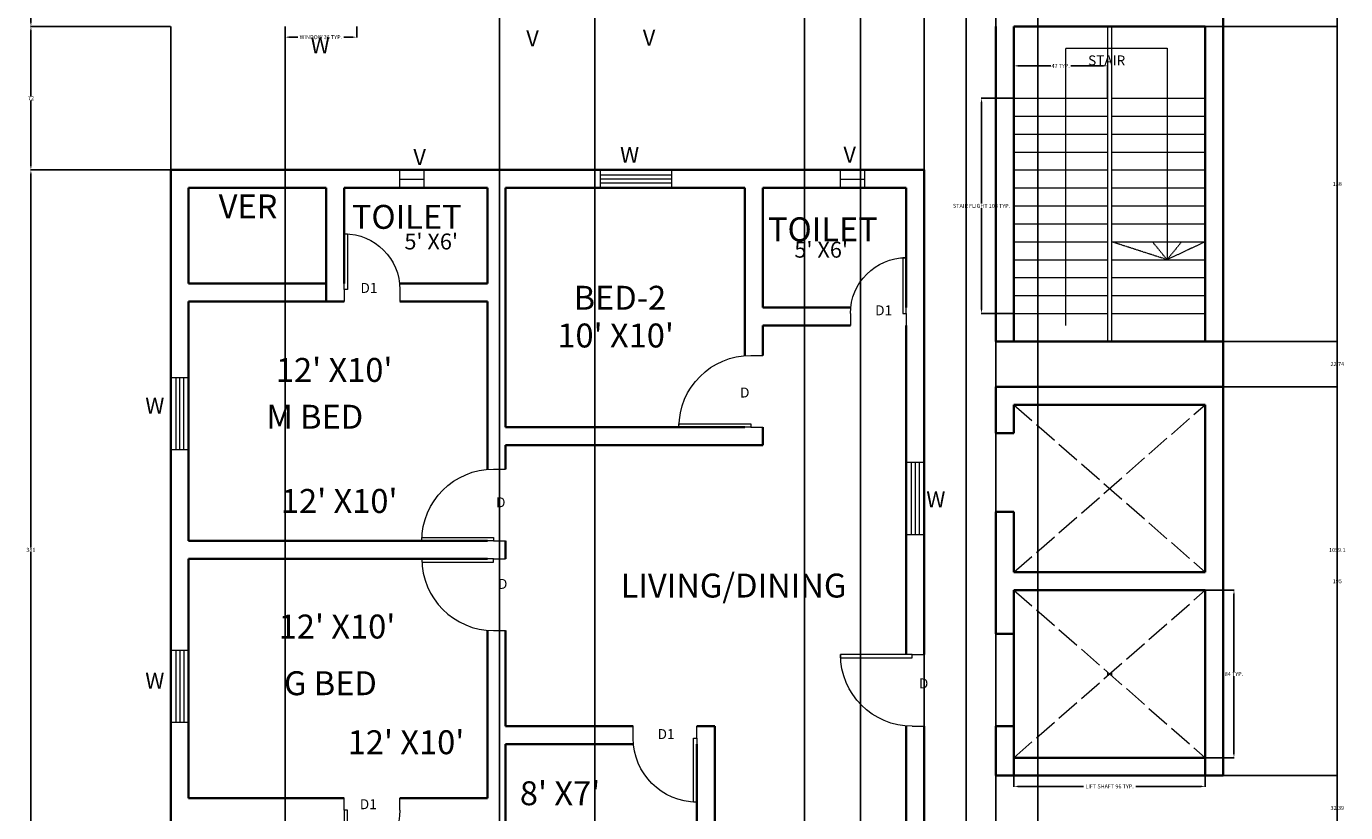
# Model space of a CAD drawing. Units: inches. Extents: x 168 to 831, y 504 to 1681.
# Tile 2 of 3: x 169 to 831, y 961 to 1355. Entities that reach past the tile are written whole.
import ezdxf

# ---------------------------------------------------------------- set-up
doc = ezdxf.new("R2010")
doc.units = ezdxf.units.IN
doc.header["$MEASUREMENT"] = 0
doc.linetypes.add('ACAD_ISO02W100', pattern=[15, 12, -3])
doc.linetypes.add('HIDDEN', pattern=[0.375, 0.25, -0.125])
for name, color, linetype, lineweight in [('A-ANNO-DIMS', 2, 'Continuous', 13), ('A-ANNO-TEXT', 7, 'Continuous', 18), ('A-AREA-IDEN', 7, 'Continuous', 18), ('A-DOOR', 3, 'Continuous', 18), ('A-FLOR-EVTR', 7, 'Continuous', 35), ('A-FLOR-EVTR-SYMB', 8, 'ACAD_ISO02W100', 13), ('A-FLOR-STRS', 8, 'Continuous', 18), ('A-FLOR-STRS-PATH', 2, 'HIDDEN', 13), ('A-GLAZ', 4, 'Continuous', 18), ('A-WALL', 7, 'Continuous', 35)]:
    doc.layers.add(name, color=color, linetype=linetype, lineweight=lineweight)
doc.styles.get("Standard").update_dxf_attribs({"font": 'arial.ttf'})
doc.dimstyles.get("Standard").update_dxf_attribs({"dimtxt": 2, "dimasz": 2, "dimexe": 0.18, "dimexo": 0.0625, "dimgap": 0.09, "dimtad": 0, "dimtih": 1, "dimtoh": 1, "dimdec": 0, "dimzin": 0, "dimdsep": 46, "dimlunit": 3, "dimtxsty": 'Standard', "dimcen": 0.09, "dimadec": 0, "dimazin": 0, "dimtfac": 1, "dimtdec": 0, "dimtofl": 0, "dimtmove": 0, "dimatfit": 3, "dimfxl": 1, "dimtolj": 1, "dimtzin": 0, "dimarcsym": 0})

# ---------------------------------------------------------------- blocks, each defined once
blk = doc.blocks.new('*U4')
for p, q in [((0, 0), (0, -6)), ((28, 0), (28, -6))]:
    blk.add_line(p, q)
blk.add_lwpolyline([(0, 0), (0, 28), (1.75, 28), (1.75, 0)], close=True)
blk.add_arc((0, 0), 28, 0, 90)
blk = doc.blocks.new('*U9')
for p, q in [((0, 0), (0, -6)), ((-36, 0), (-36, -6))]:
    blk.add_line(p, q)
blk.add_lwpolyline([(0, 0), (0, 36), (-1.75, 36), (-1.75, 0)], close=True)
blk.add_arc((0, 0), 36, 90, 180)
blk = doc.blocks.new('*U11')
for p, q in [((0, 0), (0, 6)), ((32, 0), (32, 6))]:
    blk.add_line(p, q)
blk.add_lwpolyline([(0, 0), (0, -32), (1.75, -32), (1.75, 0)], close=True)
blk.add_arc((0, 0), 32, 270, 0)
blk = doc.blocks.new('*U10')
for p, q in [((0, 0), (0, -6)), ((-36, 0), (-36, -6))]:
    blk.add_line(p, q)
blk.add_lwpolyline([(0, 0), (0, 36), (-1.75, 36), (-1.75, 0)], close=True)
blk.add_arc((0, 0), 36, 90, 180)
blk = doc.blocks.new('*U12')
for p, q in [((-28, 0), (-28, 6)), ((0, 0), (0, 6))]:
    blk.add_line(p, q)
blk.add_lwpolyline([(0, 0), (0, -28), (-1.75, -28), (-1.75, 0)], close=True)
blk.add_arc((0, 0), 28, 180, 270)
blk = doc.blocks.new('*U13')
for p, q in [((-28, 0), (-28, -6)), ((0, 0), (0, -6))]:
    blk.add_line(p, q)
blk.add_lwpolyline([(0, 0), (0, 28), (-1.75, 28), (-1.75, 0)], close=True)
blk.add_arc((0, 0), 28, 90, 180)
blk = doc.blocks.new('*U14')
for p, q in [((0, 0), (0, -6)), ((36, 0), (36, -6))]:
    blk.add_line(p, q)
blk.add_lwpolyline([(0, 0), (0, 36), (1.75, 36), (1.75, 0)], close=True)
blk.add_arc((0, 0), 36, 0, 90)
blk = doc.blocks.new('WIN-36IN')
for p, q in [((0, 6.5), (36, 6.5)), ((0, 4.5), (36, 4.5)), ((0, 2.5), (36, 2.5))]:
    blk.add_line(p, q)
blk.add_lwpolyline([(36, 0), (36, 9), (0, 9), (0, 0)], close=True)
blk = doc.blocks.new('VENT-12IN')
blk.add_line((0, 4.5), (12, 4.5))
blk.add_lwpolyline([(0, 0), (0, 9), (12, 9), (12, 0)], close=True)
blk = doc.blocks.new('LIFT-SHAFT-MARK-96X84')
for p, q in [((0, 0), (96, 84)), ((0, 84), (96, 0))]:
    blk.add_line(p, q)
blk = doc.blocks.new('STAIR-FLIGHT-13-TREADS')
for p, q in [((0, 108), (47, 108)), ((0, 99), (47, 99)), ((0, 90), (47, 90)), ((0, 81), (47, 81)), ((0, 72), (47, 72)), ((0, 63), (47, 63)), ((0, 54), (47, 54)), ((0, 45), (47, 45)), ((0, 36), (47, 36)), ((0, 27), (47, 27)), ((0, 18), (47, 18)), ((0, 9), (47, 9)), ((0, 0), (47, 0))]:
    blk.add_line(p, q)
blk = doc.blocks.new('*D20')
at = {"layer": 'A-ANNO-DIMS', "color": 0, "lineweight": -2, "transparency": 16777216}
for p, q in [((299.21, 1354.98), (299.21, 1349.46)), ((335.21, 1354.98), (335.21, 1349.46)), ((301.21, 1349.64), (305.7, 1349.64)), ((333.21, 1349.64), (328.73, 1349.64))]:
    blk.add_line(p, q, dxfattribs=at)
at = {"layer": 'A-ANNO-DIMS', "color": 0, "transparency": 16777216}
for points in [[(301.21, 1349.97), (301.21, 1349.31), (299.21, 1349.64)], [(333.21, 1349.97), (333.21, 1349.31), (335.21, 1349.64)]]:
    blk.add_solid(points, dxfattribs=at)
at = {"layer": 'Defpoints', "color": 0, "transparency": 16777216}
for p in [(299.21, 1355.04), (335.21, 1355.04), (335.21, 1349.64)]:
    blk.add_point(p, dxfattribs=at)
at = {"layer": 'A-ANNO-DIMS', "color": 0, "transparency": 16777216, "insert": (317.21, 1349.64), "char_height": 2, "attachment_point": 5}
blk.add_mtext('\\A1;WINDOW 36 TYP.', dxfattribs=at)
blk = doc.blocks.new('*D26')
at = {"layer": 'A-ANNO-DIMS', "color": 0, "lineweight": -2, "transparency": 16777216}
for p, q in [((664.86, 988.24), (664.86, 973.72)), ((760.86, 988.24), (760.86, 973.72)), ((666.86, 973.9), (699.72, 973.9)), ((758.86, 973.9), (726, 973.9))]:
    blk.add_line(p, q, dxfattribs=at)
at = {"layer": 'A-ANNO-DIMS', "color": 0, "transparency": 16777216}
for points in [[(666.86, 974.23), (666.86, 973.57), (664.86, 973.9)], [(758.86, 974.23), (758.86, 973.57), (760.86, 973.9)]]:
    blk.add_solid(points, dxfattribs=at)
at = {"layer": 'Defpoints', "color": 0, "transparency": 16777216}
for p in [(664.86, 988.3), (760.86, 988.3), (760.86, 973.9)]:
    blk.add_point(p, dxfattribs=at)
at = {"layer": 'A-ANNO-DIMS', "color": 0, "transparency": 16777216, "insert": (712.86, 973.9), "char_height": 2, "attachment_point": 5}
blk.add_mtext('\\A1;LIFT SHAFT 96 TYP.', dxfattribs=at)
blk = doc.blocks.new('*D27')
at = {"layer": 'A-ANNO-DIMS', "color": 0, "lineweight": -2, "transparency": 16777216}
for p, q in [((760.93, 1072.3), (775.44, 1072.3)), ((775.26, 1070.3), (775.26, 1031.41)), ((775.26, 990.3), (775.26, 1029.19)), ((760.93, 988.3), (775.44, 988.3))]:
    blk.add_line(p, q, dxfattribs=at)
at = {"layer": 'A-ANNO-DIMS', "color": 0, "transparency": 16777216}
for points in [[(774.93, 1070.3), (775.6, 1070.3), (775.26, 1072.3)], [(774.93, 990.3), (775.6, 990.3), (775.26, 988.3)]]:
    blk.add_solid(points, dxfattribs=at)
at = {"layer": 'Defpoints', "color": 0, "transparency": 16777216}
for p in [(760.86, 1072.3), (775.26, 1072.3), (760.86, 988.3)]:
    blk.add_point(p, dxfattribs=at)
at = {"layer": 'A-ANNO-DIMS', "color": 0, "transparency": 16777216, "insert": (775.26, 1030.3), "char_height": 2, "attachment_point": 5}
blk.add_mtext('\\A1;84 TYP.', dxfattribs=at)
blk = doc.blocks.new('*D28')
at = {"layer": 'A-ANNO-DIMS', "color": 0, "lineweight": -2, "transparency": 16777216}
for p, q in [((664.8, 1319.04), (648.48, 1319.04)), ((648.66, 1317.04), (648.66, 1266.16)), ((648.66, 1213.04), (648.66, 1263.91)), ((664.8, 1211.04), (648.48, 1211.04))]:
    blk.add_line(p, q, dxfattribs=at)
at = {"layer": 'A-ANNO-DIMS', "color": 0, "transparency": 16777216}
for points in [[(648.33, 1317.04), (649, 1317.04), (648.66, 1319.04)], [(648.33, 1213.04), (649, 1213.04), (648.66, 1211.04)]]:
    blk.add_solid(points, dxfattribs=at)
at = {"layer": 'Defpoints', "color": 0, "transparency": 16777216}
for p in [(648.66, 1319.04), (664.86, 1319.04), (664.86, 1211.04)]:
    blk.add_point(p, dxfattribs=at)
at = {"layer": 'A-ANNO-DIMS', "color": 0, "transparency": 16777216, "insert": (648.66, 1265.04), "char_height": 2, "attachment_point": 5}
blk.add_mtext('\\A1;STAIR FLIGHT 108 TYP.', dxfattribs=at)
blk = doc.blocks.new('*D29')
at = {"layer": 'A-ANNO-DIMS', "color": 0, "lineweight": -2, "transparency": 16777216}
for p, q in [((664.86, 1319.1), (664.86, 1335.42)), ((666.86, 1335.24), (683.37, 1335.24)), ((709.86, 1335.24), (693.36, 1335.24)), ((711.86, 1319.1), (711.86, 1335.42))]:
    blk.add_line(p, q, dxfattribs=at)
at = {"layer": 'A-ANNO-DIMS', "color": 0, "transparency": 16777216}
for points in [[(666.86, 1335.57), (666.86, 1334.91), (664.86, 1335.24)], [(709.86, 1335.57), (709.86, 1334.91), (711.86, 1335.24)]]:
    blk.add_solid(points, dxfattribs=at)
at = {"layer": 'Defpoints', "color": 0, "transparency": 16777216}
for p in [(711.86, 1335.24), (664.86, 1319.04), (711.86, 1319.04)]:
    blk.add_point(p, dxfattribs=at)
at = {"layer": 'A-ANNO-DIMS', "color": 0, "transparency": 16777216, "insert": (688.36, 1335.24), "char_height": 2, "attachment_point": 5}
blk.add_mtext('\\A1;47 TYP.', dxfattribs=at)
blk = doc.blocks.new('*D31')
at = {"layer": 'A-ANNO-DIMS', "color": 0, "lineweight": -2, "transparency": 16777216}
for p, q in [((769.93, 1622.04), (827.29, 1622.04)), ((827.11, 1620.04), (827.11, 1093.58)), ((827.11, 564.91), (827.11, 1091.36)), ((769.93, 562.91), (827.29, 562.91))]:
    blk.add_line(p, q, dxfattribs=at)
at = {"layer": 'A-ANNO-DIMS', "color": 0, "transparency": 16777216}
for points in [[(826.78, 1620.04), (827.45, 1620.04), (827.11, 1622.04)], [(826.78, 564.91), (827.45, 564.91), (827.11, 562.91)]]:
    blk.add_solid(points, dxfattribs=at)
at = {"layer": 'Defpoints', "color": 0, "transparency": 16777216}
for p in [(769.86, 1622.04), (827.11, 1622.04), (769.86, 562.91)]:
    blk.add_point(p, dxfattribs=at)
at = {"layer": 'A-ANNO-DIMS', "color": 0, "transparency": 16777216, "insert": (827.11, 1092.47), "char_height": 2, "attachment_point": 5}
blk.add_mtext('\\A1;1059.1', dxfattribs=at)
blk = doc.blocks.new('*D34')
at = {"layer": 'A-ANNO-DIMS', "color": 0, "lineweight": -2, "transparency": 16777216}
for p, q in [((241.8, 1283.04), (171.56, 1283.04)), ((171.74, 1281.04), (171.74, 1093.65)), ((171.74, 904.04), (171.74, 1091.43)), ((241.8, 902.04), (171.56, 902.04))]:
    blk.add_line(p, q, dxfattribs=at)
at = {"layer": 'A-ANNO-DIMS', "color": 0, "transparency": 16777216}
for points in [[(171.41, 1281.04), (172.08, 1281.04), (171.74, 1283.04)], [(171.41, 904.04), (172.08, 904.04), (171.74, 902.04)]]:
    blk.add_solid(points, dxfattribs=at)
at = {"layer": 'Defpoints', "color": 0, "transparency": 16777216}
for p in [(171.74, 1283.04), (241.86, 1283.04), (241.86, 902.04)]:
    blk.add_point(p, dxfattribs=at)
at = {"layer": 'A-ANNO-DIMS', "color": 0, "transparency": 16777216, "insert": (171.74, 1092.54), "char_height": 2, "attachment_point": 5}
blk.add_mtext('\\A1;381', dxfattribs=at)
blk = doc.blocks.new('*D35')
at = {"layer": 'A-ANNO-DIMS', "color": 0, "lineweight": -2, "transparency": 16777216}
for p, q in [((241.8, 1355.04), (171.56, 1355.04)), ((171.74, 1353.04), (171.74, 1320.13)), ((171.74, 1285.04), (171.74, 1317.94)), ((241.8, 1283.04), (171.56, 1283.04))]:
    blk.add_line(p, q, dxfattribs=at)
at = {"layer": 'A-ANNO-DIMS', "color": 0, "transparency": 16777216}
for points in [[(171.41, 1353.04), (172.08, 1353.04), (171.74, 1355.04)], [(171.41, 1285.04), (172.08, 1285.04), (171.74, 1283.04)]]:
    blk.add_solid(points, dxfattribs=at)
at = {"layer": 'Defpoints', "color": 0, "transparency": 16777216}
for p in [(171.74, 1355.04), (241.86, 1355.04), (241.86, 1283.04)]:
    blk.add_point(p, dxfattribs=at)
at = {"layer": 'A-ANNO-DIMS', "color": 0, "transparency": 16777216, "insert": (171.74, 1319.04), "char_height": 2, "attachment_point": 5}
blk.add_mtext('\\A1;72', dxfattribs=at)
blk = doc.blocks.new('*D36')
at = {"layer": 'A-ANNO-DIMS', "color": 0, "lineweight": -2, "transparency": 16777216}
for p, q in [((346.8, 1622.04), (171.56, 1622.04)), ((171.74, 1620.04), (171.74, 1489.65)), ((171.74, 1357.04), (171.74, 1487.43)), ((241.8, 1355.04), (171.56, 1355.04))]:
    blk.add_line(p, q, dxfattribs=at)
at = {"layer": 'A-ANNO-DIMS', "color": 0, "transparency": 16777216}
for points in [[(171.41, 1620.04), (172.08, 1620.04), (171.74, 1622.04)], [(171.41, 1357.04), (172.08, 1357.04), (171.74, 1355.04)]]:
    blk.add_solid(points, dxfattribs=at)
at = {"layer": 'Defpoints', "color": 0, "transparency": 16777216}
for p in [(171.74, 1622.04), (346.86, 1622.04), (241.86, 1355.04)]:
    blk.add_point(p, dxfattribs=at)
at = {"layer": 'A-ANNO-DIMS', "color": 0, "transparency": 16777216, "insert": (171.74, 1488.54), "char_height": 2, "attachment_point": 5}
blk.add_mtext('\\A1;267', dxfattribs=at)
blk = doc.blocks.new('*D40')
at = {"layer": 'A-ANNO-DIMS', "color": 0, "lineweight": -2, "transparency": 16777216}
for p, q in [((619.86, 902.1), (619.86, 1679.47)), ((621.86, 1679.29), (636.34, 1679.29)), ((653.86, 1679.29), (639.38, 1679.29)), ((655.86, 946.97), (655.86, 1679.47))]:
    blk.add_line(p, q, dxfattribs=at)
at = {"layer": 'A-ANNO-DIMS', "color": 0, "transparency": 16777216}
for points in [[(621.86, 1679.62), (621.86, 1678.96), (619.86, 1679.29)], [(653.86, 1679.62), (653.86, 1678.96), (655.86, 1679.29)]]:
    blk.add_solid(points, dxfattribs=at)
at = {"layer": 'Defpoints', "color": 0, "transparency": 16777216}
for p in [(655.86, 1679.29), (655.86, 946.91), (619.86, 902.04)]:
    blk.add_point(p, dxfattribs=at)
at = {"layer": 'A-ANNO-DIMS', "color": 0, "transparency": 16777216, "insert": (637.86, 1679.29), "char_height": 2, "attachment_point": 5}
blk.add_mtext('\\A1;36', dxfattribs=at)
blk = doc.blocks.new('*D43')
at = {"layer": 'A-ANNO-DIMS', "color": 0, "lineweight": -2, "transparency": 16777216}
for p, q in [((769.93, 979.3), (827.29, 979.3)), ((827.11, 977.3), (827.11, 964.22)), ((827.11, 948.91), (827.11, 961.99)), ((769.93, 946.91), (827.29, 946.91))]:
    blk.add_line(p, q, dxfattribs=at)
at = {"layer": 'A-ANNO-DIMS', "color": 0, "transparency": 16777216}
for points in [[(826.78, 977.3), (827.45, 977.3), (827.11, 979.3)], [(826.78, 948.91), (827.45, 948.91), (827.11, 946.91)]]:
    blk.add_solid(points, dxfattribs=at)
at = {"layer": 'Defpoints', "color": 0, "transparency": 16777216}
for p in [(769.86, 979.3), (827.11, 979.3), (769.86, 946.91)]:
    blk.add_point(p, dxfattribs=at)
at = {"layer": 'A-ANNO-DIMS', "color": 0, "transparency": 16777216, "insert": (827.11, 963.1), "char_height": 2, "attachment_point": 5}
blk.add_mtext('\\A1;32.39', dxfattribs=at)
blk = doc.blocks.new('*D44')
at = {"layer": 'A-ANNO-DIMS', "color": 0, "lineweight": -2, "transparency": 16777216}
for p, q in [((769.93, 1174.3), (827.29, 1174.3)), ((827.11, 1172.3), (827.11, 1077.91)), ((827.11, 981.3), (827.11, 1075.69)), ((769.93, 979.3), (827.29, 979.3))]:
    blk.add_line(p, q, dxfattribs=at)
at = {"layer": 'A-ANNO-DIMS', "color": 0, "transparency": 16777216}
for points in [[(826.78, 1172.3), (827.45, 1172.3), (827.11, 1174.3)], [(826.78, 981.3), (827.45, 981.3), (827.11, 979.3)]]:
    blk.add_solid(points, dxfattribs=at)
at = {"layer": 'Defpoints', "color": 0, "transparency": 16777216}
for p in [(769.86, 1174.3), (827.11, 1174.3), (769.86, 979.3)]:
    blk.add_point(p, dxfattribs=at)
at = {"layer": 'A-ANNO-DIMS', "color": 0, "transparency": 16777216, "insert": (827.11, 1076.8), "char_height": 2, "attachment_point": 5}
blk.add_mtext('\\A1;195', dxfattribs=at)
blk = doc.blocks.new('*D45')
at = {"layer": 'A-ANNO-DIMS', "color": 0, "lineweight": -2, "transparency": 16777216}
for p, q in [((769.93, 1197.04), (827.29, 1197.04)), ((827.11, 1195.04), (827.11, 1186.76)), ((827.11, 1176.3), (827.11, 1184.58)), ((769.93, 1174.3), (827.29, 1174.3))]:
    blk.add_line(p, q, dxfattribs=at)
at = {"layer": 'A-ANNO-DIMS', "color": 0, "transparency": 16777216}
for points in [[(826.78, 1195.04), (827.45, 1195.04), (827.11, 1197.04)], [(826.78, 1176.3), (827.45, 1176.3), (827.11, 1174.3)]]:
    blk.add_solid(points, dxfattribs=at)
at = {"layer": 'Defpoints', "color": 0, "transparency": 16777216}
for p in [(769.86, 1197.04), (827.11, 1197.04), (769.86, 1174.3)]:
    blk.add_point(p, dxfattribs=at)
at = {"layer": 'A-ANNO-DIMS', "color": 0, "transparency": 16777216, "insert": (827.11, 1185.67), "char_height": 2, "attachment_point": 5}
blk.add_mtext('\\A1;22.74', dxfattribs=at)
blk = doc.blocks.new('*D46')
at = {"layer": 'A-ANNO-DIMS', "color": 0, "lineweight": -2, "transparency": 16777216}
for p, q in [((760.93, 1355.04), (827.29, 1355.04)), ((827.11, 1353.04), (827.11, 1277.15)), ((827.11, 1199.04), (827.11, 1274.93)), ((769.93, 1197.04), (827.29, 1197.04))]:
    blk.add_line(p, q, dxfattribs=at)
at = {"layer": 'A-ANNO-DIMS', "color": 0, "transparency": 16777216}
for points in [[(826.78, 1353.04), (827.45, 1353.04), (827.11, 1355.04)], [(826.78, 1199.04), (827.45, 1199.04), (827.11, 1197.04)]]:
    blk.add_solid(points, dxfattribs=at)
at = {"layer": 'Defpoints', "color": 0, "transparency": 16777216}
for p in [(760.86, 1355.04), (827.11, 1355.04), (769.86, 1197.04)]:
    blk.add_point(p, dxfattribs=at)
at = {"layer": 'A-ANNO-DIMS', "color": 0, "transparency": 16777216, "insert": (827.11, 1276.04), "char_height": 2, "attachment_point": 5}
blk.add_mtext('\\A1;158', dxfattribs=at)
blk = doc.blocks.new('*D47')
at = {"layer": 'A-ANNO-DIMS', "color": 0, "lineweight": -2, "transparency": 16777216}
for p, q in [((559.86, 1483.98), (559.86, 505.48)), ((587.86, 1483.98), (587.86, 505.48)), ((561.86, 505.66), (572.32, 505.66)), ((585.86, 505.66), (575.4, 505.66))]:
    blk.add_line(p, q, dxfattribs=at)
at = {"layer": 'A-ANNO-DIMS', "color": 0, "transparency": 16777216}
for points in [[(561.86, 505.99), (561.86, 505.32), (559.86, 505.66)], [(585.86, 505.99), (585.86, 505.32), (587.86, 505.66)]]:
    blk.add_solid(points, dxfattribs=at)
at = {"layer": 'Defpoints', "color": 0, "transparency": 16777216}
for p in [(559.86, 1484.04), (587.86, 1484.04), (587.86, 505.66)]:
    blk.add_point(p, dxfattribs=at)
at = {"layer": 'A-ANNO-DIMS', "color": 0, "transparency": 16777216, "insert": (573.86, 505.66), "char_height": 2, "attachment_point": 5}
blk.add_mtext('\\A1;28', dxfattribs=at)
blk = doc.blocks.new('*D48')
at = {"layer": 'A-ANNO-DIMS', "color": 0, "lineweight": -2, "transparency": 16777216}
for p, q in [((640.86, 1483.98), (640.86, 505.48)), ((676.86, 1483.98), (676.86, 505.48)), ((642.86, 505.66), (657.34, 505.66)), ((674.86, 505.66), (660.38, 505.66))]:
    blk.add_line(p, q, dxfattribs=at)
at = {"layer": 'A-ANNO-DIMS', "color": 0, "transparency": 16777216}
for points in [[(642.86, 505.99), (642.86, 505.32), (640.86, 505.66)], [(674.86, 505.99), (674.86, 505.32), (676.86, 505.66)]]:
    blk.add_solid(points, dxfattribs=at)
at = {"layer": 'Defpoints', "color": 0, "transparency": 16777216}
for p in [(640.86, 1484.04), (676.86, 1484.04), (676.86, 505.66)]:
    blk.add_point(p, dxfattribs=at)
at = {"layer": 'A-ANNO-DIMS', "color": 0, "transparency": 16777216, "insert": (658.86, 505.66), "char_height": 2, "attachment_point": 5}
blk.add_mtext('\\A1;36', dxfattribs=at)
blk = doc.blocks.new('*D52')
at = {"layer": 'A-ANNO-DIMS', "color": 0, "lineweight": -2, "transparency": 16777216}
for p, q in [((406.86, 1612.98), (406.86, 505.48)), ((454.72, 1612.98), (454.72, 505.48)), ((408.86, 505.66), (427.29, 505.66)), ((452.72, 505.66), (434.3, 505.66))]:
    blk.add_line(p, q, dxfattribs=at)
at = {"layer": 'A-ANNO-DIMS', "color": 0, "transparency": 16777216}
for points in [[(408.86, 505.99), (408.86, 505.32), (406.86, 505.66)], [(452.72, 505.99), (452.72, 505.32), (454.72, 505.66)]]:
    blk.add_solid(points, dxfattribs=at)
at = {"layer": 'Defpoints', "color": 0, "transparency": 16777216}
for p in [(406.86, 1613.04), (454.72, 1613.04), (454.72, 505.66)]:
    blk.add_point(p, dxfattribs=at)
at = {"layer": 'A-ANNO-DIMS', "color": 0, "transparency": 16777216, "insert": (430.79, 505.66), "char_height": 2, "attachment_point": 5}
blk.add_mtext('\\A1;47.86', dxfattribs=at)
blk = doc.blocks.new('*D53')
at = {"layer": 'A-ANNO-DIMS', "color": 0, "lineweight": -2, "transparency": 16777216}
for p, q in [((241.86, 1354.98), (241.86, 505.48)), ((299.21, 1354.98), (299.21, 505.48)), ((243.86, 505.66), (267.07, 505.66)), ((297.21, 505.66), (274.01, 505.66))]:
    blk.add_line(p, q, dxfattribs=at)
at = {"layer": 'A-ANNO-DIMS', "color": 0, "transparency": 16777216}
for points in [[(243.86, 505.99), (243.86, 505.32), (241.86, 505.66)], [(297.21, 505.99), (297.21, 505.32), (299.21, 505.66)]]:
    blk.add_solid(points, dxfattribs=at)
at = {"layer": 'Defpoints', "color": 0, "transparency": 16777216}
for p in [(241.86, 1355.04), (299.21, 1355.04), (299.21, 505.66)]:
    blk.add_point(p, dxfattribs=at)
at = {"layer": 'A-ANNO-DIMS', "color": 0, "transparency": 16777216, "insert": (270.54, 505.66), "char_height": 2, "attachment_point": 5}
blk.add_mtext('\\A1;57.35', dxfattribs=at)

msp = doc.modelspace()

# ---------------------------------------------------------------- linework, layer by layer
at = {"layer": 'A-FLOR-EVTR'}
for p, q in [((655.863, 1174.3), (769.863, 1174.3)), ((655.863, 1174.3), (655.863, 1150.97)), ((660.363, 1174.3), (765.363, 1174.3)), ((664.863, 1165.3), (760.863, 1165.3)), ((664.863, 1165.3), (664.863, 1150.97)), ((760.863, 1165.3), (760.863, 1081.3)), ((664.863, 1150.97), (655.863, 1150.97)), ((664.863, 1111.663), (655.863, 1111.663)), ((655.863, 1111.663), (655.863, 1050.464)), ((664.863, 1111.663), (664.863, 1111.663)), ((664.863, 1111.663), (664.863, 1081.3)), ((664.863, 1081.3), (760.863, 1081.3)), ((664.863, 1072.3), (760.863, 1072.3)), ((664.863, 1072.3), (664.863, 1050.464)), ((760.863, 1072.3), (760.863, 979.3)), ((664.863, 1050.464), (655.863, 1050.464)), ((664.863, 1050.464), (664.863, 979.3)), ((655.863, 1004.019), (664.863, 1004.019)), ((655.863, 1004.019), (655.863, 979.3)), ((664.863, 988.3), (760.863, 988.3)), ((655.863, 979.3), (769.863, 979.3))]:
    msp.add_line(p, q, dxfattribs=at)
at = {"layer": 'A-FLOR-EVTR-SYMB'}
for p, q in [((711.863, 1031.175), (711.863, 1029.425)), ((713.863, 1031.175), (713.863, 1029.425))]:
    msp.add_line(p, q, dxfattribs=at)
at = {"layer": 'A-FLOR-STRS'}
for p, q in [((711.863, 1355.039), (711.863, 1197.039)), ((713.863, 1355.039), (713.863, 1197.039))]:
    msp.add_line(p, q, dxfattribs=at)
at = {"layer": 'A-FLOR-STRS-PATH'}
for p, q in [((690.882, 1205.035), (690.882, 1344.036)), ((690.882, 1344.036), (741.716, 1344.036)), ((741.716, 1344.036), (741.716, 1238.039)), ((741.716, 1238.039), (713.863, 1247.039)), ((713.863, 1247.039), (760.863, 1247.039)), ((741.716, 1238.039), (734.35, 1247.039)), ((734.35, 1247.039), (749.046, 1247.039)), ((749.046, 1247.039), (741.716, 1238.039)), ((760.863, 1247.039), (741.716, 1238.039))]:
    msp.add_line(p, q, dxfattribs=at)
at = {"layer": 'A-WALL'}
for p, q in [((769.863, 1622.039), (769.863, 1197.039)), ((769.863, 1406.112), (769.863, 979.3)), ((655.863, 1355.039), (655.863, 1197.039)), ((664.863, 1355.039), (664.863, 1197.039)), ((664.863, 1355.039), (760.863, 1355.039)), ((760.863, 1355.039), (760.863, 1197.039)), ((241.863, 1283.039), (619.863, 1283.039)), ((241.863, 902.039), (241.863, 1283.039)), ((619.863, 1283.039), (619.863, 1040.039)), ((250.863, 1274.039), (319.863, 1274.039)), ((250.863, 1226.039), (250.863, 1274.039)), ((319.863, 1274.039), (319.863, 1217.039)), ((328.863, 1274.039), (328.863, 1226.039)), ((328.863, 1274.039), (400.863, 1274.039)), ((400.863, 1274.039), (400.863, 1226.039)), ((409.863, 1274.039), (409.863, 1154.039)), ((409.863, 1274.039), (529.863, 1274.039)), ((529.863, 1274.039), (529.863, 1189.913)), ((538.863, 1274.039), (610.863, 1274.039)), ((538.863, 1274.039), (538.863, 1214.039)), ((610.863, 1274.039), (610.863, 1214.039)), ((250.863, 1226.039), (319.863, 1226.039)), ((356.702, 1226.039), (400.863, 1226.039)), ((250.863, 1217.039), (328.863, 1217.039)), ((250.863, 1097.039), (250.863, 1217.039)), ((356.863, 1217.039), (400.863, 1217.039)), ((400.863, 1217.039), (400.863, 1132.914)), ((538.863, 1214.039), (583.025, 1214.039)), ((538.863, 1205.039), (582.863, 1205.039)), ((538.863, 1205.039), (538.863, 1190.038)), ((610.863, 1205.039), (610.863, 1040.039)), ((655.863, 1197.039), (664.863, 1197.039)), ((664.863, 1197.039), (760.863, 1197.039)), ((760.863, 1197.039), (769.863, 1197.039)), ((409.863, 1154.039), (529.863, 1154.039)), ((538.863, 1154.038), (538.863, 1145.039)), ((409.863, 1145.039), (538.863, 1145.039)), ((409.863, 1145.039), (409.863, 1133.039)), ((250.863, 1097.039), (400.863, 1097.039)), ((409.863, 1097.039), (409.863, 1088.039)), ((250.863, 1088.039), (400.863, 1088.039)), ((250.863, 968.039), (250.863, 1088.039)), ((400.863, 1052.164), (400.863, 968.039)), ((409.863, 1052.039), (409.863, 1004.039)), ((409.863, 1004.039), (473.863, 1004.039)), ((505.863, 1004.039), (514.863, 1004.039)), ((514.863, 1004.039), (514.863, 911.039)), ((610.863, 1004.164), (610.863, 911.039)), ((619.863, 1004.039), (619.863, 902.039)), ((409.863, 995.039), (474.004, 995.039)), ((409.863, 995.039), (409.863, 911.039)), ((505.863, 995.039), (505.863, 911.039)), ((250.863, 968.039), (328.863, 968.039)), ((356.863, 968.039), (400.863, 968.039))]:
    msp.add_line(p, q, dxfattribs=at)

# ---------------------------------------------------------------- block references
at = {"layer": 'A-DOOR', "xscale": -1}
for name, p in [('*U13', (328.863, 1223.039)), ('*U4', (610.863, 1211.039)), ('*U11', (505.863, 998.039)), ('*U12', (328.863, 962.039))]:
    msp.add_blockref(name, p, dxfattribs=at)
at = {"layer": 'A-DOOR', "xscale": -1, "rotation": 90}
for name, p in [('*U9', (532.863, 1154.038)), ('*U10', (403.863, 1097.039)), ('*U14', (613.863, 1040.039))]:
    msp.add_blockref(name, p, dxfattribs=at)
at = {"layer": 'A-DOOR', "rotation": 90.00000000000003}
msp.add_blockref('*U10', (403.863, 1088.039), dxfattribs=at)
at = {"layer": 'A-FLOR-EVTR-SYMB'}
for p in [(664.863, 1081.3), (664.863, 988.3)]:
    msp.add_blockref('LIFT-SHAFT-MARK-96X84', p, dxfattribs=at)
at = {"layer": 'A-FLOR-STRS'}
for p in [(664.863, 1211.039), (713.863, 1211.039)]:
    msp.add_blockref('STAIR-FLIGHT-13-TREADS', p, dxfattribs=at)
at = {"layer": 'A-GLAZ'}
for name, p in [('VENT-12IN', (356.86, 1273.914)), ('WIN-36IN', (457.238, 1274.039)), ('WIN-36IN', (457.238, 1274.039)), ('VENT-12IN', (577.884, 1273.953))]:
    msp.add_blockref(name, p, dxfattribs=at)
for p, rotation in [((241.868, 1178.789), 270.0000000000007), ((241.868, 1178.789), 270.0000000000007), ((610.865, 1136.266), 270.0000000000007), ((610.865, 1136.266), 270.0000000000007), ((241.887, 1042.039), 270.0000000000009), ((241.887, 1042.039), 270.0000000000009)]:
    msp.add_blockref('WIN-36IN', p, dxfattribs=dict(at, rotation=rotation))

# ---------------------------------------------------------------- texts
at = {"layer": 'A-ANNO-DIMS', "attachment_point": 1}
for s, width, insert, char_height in [("5' X6'", 59.10581, (359.105, 1251.166), 8), ("5' X6'", 59.10581, (554.752, 1247.047), 8), ("10' X10'", 157.93148, (435.837, 1206.025), 12), ("12' X10'", 157.93148, (294.65, 1188.759), 12), ("12' X10'", 157.93148, (297.176, 1123.038), 12), ("12' X10'", 157.93148, (296.058, 1060.064), 12), ("12' X10'", 157.93148, (330.67, 1002.044), 12), ("8' X7'", 157.93148, (417.032, 976.459), 12)]:
    msp.add_mtext_dynamic_manual_height_columns(s, width=width, gutter_width=1, heights=[0], dxfattribs=dict(at, insert=insert, char_height=char_height))
at = {"layer": 'A-ANNO-TEXT', "attachment_point": 1}
for s, width, insert, char_height in [('V', 20.00841, (420.236, 1353.048), 8), ('V', 20.00841, (478.709, 1353.417), 8), ('W', 57.92772, (312.069, 1349.526), 8), ('V', 20.00841, (363.612, 1293.52), 8), ('W', 57.92772, (467.299, 1294.636), 8), ('V', 20.00841, (579.353, 1294.746), 8), ('D1', 11.24528, (337.081, 1226.375), 5), ('D1', 11.24528, (595.275, 1215.145), 5), ('D', 11.24528, (527.521, 1173.924), 5), ('W', 57.92772, (229.115, 1168.885), 8), ('D', 11.24528, (405.11, 1118.86), 5), ('W', 57.92772, (620.918, 1121.82), 8), ('D', 11.24528, (406.078, 1077.95), 5), ('W', 57.92772, (229.115, 1030.901), 8), ('D', 11.24528, (617.248, 1028.022), 5), ('D1', 11.24528, (486.147, 1002.644), 5), ('D1', 11.24528, (336.758, 967.464), 5)]:
    msp.add_mtext_dynamic_manual_height_columns(s, width=width, gutter_width=1, heights=[0], dxfattribs=dict(at, insert=insert, char_height=char_height))
at = {"layer": 'A-AREA-IDEN', "attachment_point": 1}
for s, width, insert, char_height in [('STAIR', 11.78067, (702.083, 1340.477), 5), ('VER', 54.54242, (265.944, 1270.765), 12), ('TOILET', 54.54242, (332.756, 1265.515), 12), ('TOILET', 54.54242, (332.756, 1265.515), 12), ('TOILET', 54.54242, (541.514, 1259.261), 12), ('BED-2', 54.54242, (443.993, 1224.938), 12), ('M BED', 54.54242, (289.837, 1165.27), 12), ('LIVING/DINING', 54.54242, (467.585, 1080.614), 12), ('G BED', 54.54242, (298.694, 1031.638), 12)]:
    msp.add_mtext_dynamic_manual_height_columns(s, width=width, gutter_width=1, heights=[0], dxfattribs=dict(at, insert=insert, char_height=char_height))

# ---------------------------------------------------------------- dimensions: what is measured, and where the dimension line sits
at = {"layer": 'A-ANNO-DIMS'}
for base, p1, p2, override, picture, middle in [((655.863, 1679.289), (619.863, 902.039), (655.863, 946.908), {"dimdec": 0, "dimlfac": 1, "dimrnd": 0, "dimzin": 0, "dimdsep": 46, "dimlunit": 2}, '*D40', (637.863, 1679.289)), ((454.72, 505.658), (406.863, 1613.039), (454.72, 1613.039), {"dimdec": 2, "dimlfac": 1, "dimrnd": 0, "dimzin": 0, "dimdsep": 46, "dimlunit": 2}, '*D52', (430.792, 505.658)), ((587.863, 505.658), (559.863, 1484.039), (587.863, 1484.039), {"dimdec": 0, "dimlfac": 1, "dimrnd": 0, "dimzin": 0, "dimdsep": 46, "dimlunit": 2}, '*D47', (573.863, 505.658)), ((676.863, 505.658), (640.863, 1484.039), (676.863, 1484.039), {"dimdec": 0, "dimlfac": 1, "dimrnd": 0, "dimzin": 0, "dimdsep": 46, "dimlunit": 2}, '*D48', (658.863, 505.658)), ((299.213, 505.658), (241.863, 1355.039), (299.213, 1355.039), {"dimdec": 2, "dimlfac": 1, "dimrnd": 0, "dimzin": 0, "dimdsep": 46, "dimlunit": 2}, '*D53', (270.538, 505.658))]:
    dim = msp.add_linear_dim(base=base, p1=p1, p2=p2, dimstyle='Standard', override=override, dxfattribs=at)
    dim.commit()
    dim.dimension.update_dxf_attribs({"geometry": picture, "text_midpoint": middle})
for base, p1, p2, override, picture, middle in [((171.744, 1622.039), (241.863, 1355.039), (346.863, 1622.039), {"dimdec": 0, "dimlfac": 1, "dimrnd": 0, "dimzin": 0, "dimdsep": 46, "dimlunit": 2}, '*D36', (171.744, 1488.539)), ((827.113, 1622.039), (769.863, 562.908), (769.863, 1622.039), {"dimdec": 1, "dimlfac": 1, "dimrnd": 0, "dimzin": 0, "dimdsep": 46, "dimlunit": 2}, '*D31', (827.113, 1092.474)), ((171.744, 1355.039), (241.863, 1283.039), (241.863, 1355.039), {"dimdec": 0, "dimlfac": 1, "dimrnd": 0, "dimzin": 0, "dimdsep": 46, "dimlunit": 2}, '*D35', (171.744, 1319.039)), ((827.113, 1355.039), (769.863, 1197.039), (760.863, 1355.039), {"dimdec": 0, "dimlfac": 1, "dimrnd": 0, "dimzin": 0, "dimdsep": 46, "dimlunit": 2}, '*D46', (827.113, 1276.039)), ((171.744, 1283.039), (241.863, 902.039), (241.863, 1283.039), {"dimdec": 0, "dimlfac": 1, "dimrnd": 0, "dimzin": 0, "dimdsep": 46, "dimlunit": 2}, '*D34', (171.744, 1092.539)), ((827.113, 1197.039), (769.863, 1174.3), (769.863, 1197.039), {"dimdec": 2, "dimlfac": 1, "dimrnd": 0, "dimzin": 0, "dimdsep": 46, "dimlunit": 2}, '*D45', (827.113, 1185.669)), ((827.113, 1174.3), (769.863, 979.3), (769.863, 1174.3), {"dimdec": 0, "dimlfac": 1, "dimrnd": 0, "dimzin": 0, "dimdsep": 46, "dimlunit": 2}, '*D44', (827.113, 1076.8)), ((827.113, 979.3), (769.863, 946.908), (769.863, 979.3), {"dimdec": 2, "dimlfac": 1, "dimrnd": 0, "dimzin": 0, "dimdsep": 46, "dimlunit": 2}, '*D43', (827.113, 963.104))]:
    dim = msp.add_linear_dim(base=base, p1=p1, p2=p2, angle=90, dimstyle='Standard', override=override, dxfattribs=at)
    dim.commit()
    dim.dimension.update_dxf_attribs({"geometry": picture, "text_midpoint": middle})
for base, p1, p2, text, picture, middle in [((335.213, 1349.639), (299.213, 1355.039), (335.213, 1355.039), 'WINDOW <> TYP.', '*D20', (317.213, 1349.639)), ((711.863, 1335.239), (664.863, 1319.039), (711.863, 1319.039), '<> TYP.', '*D29', (688.363, 1335.239)), ((760.863, 973.9), (664.863, 988.3), (760.863, 988.3), 'LIFT SHAFT <> TYP.', '*D26', (712.863, 973.9))]:
    dim = msp.add_linear_dim(base=base, p1=p1, p2=p2, text=text, dimstyle='Standard', override={"dimdec": 0, "dimlfac": 1, "dimrnd": 0, "dimzin": 0, "dimdsep": 46, "dimlunit": 2}, dxfattribs=at)
    dim.commit()
    dim.dimension.update_dxf_attribs({"geometry": picture, "text_midpoint": middle})
for base, p1, p2, text, picture, middle in [((648.663, 1319.039), (664.863, 1211.039), (664.863, 1319.039), 'STAIR FLIGHT <> TYP.', '*D28', (648.663, 1265.039)), ((775.263, 1072.3), (760.863, 988.3), (760.863, 1072.3), '<> TYP.', '*D27', (775.263, 1030.3))]:
    dim = msp.add_linear_dim(base=base, p1=p1, p2=p2, angle=90, text=text, dimstyle='Standard', override={"dimdec": 0, "dimlfac": 1, "dimrnd": 0, "dimzin": 0, "dimdsep": 46, "dimlunit": 2}, dxfattribs=at)
    dim.commit()
    dim.dimension.update_dxf_attribs({"geometry": picture, "text_midpoint": middle})

doc.saveas('drawing.dxf')
